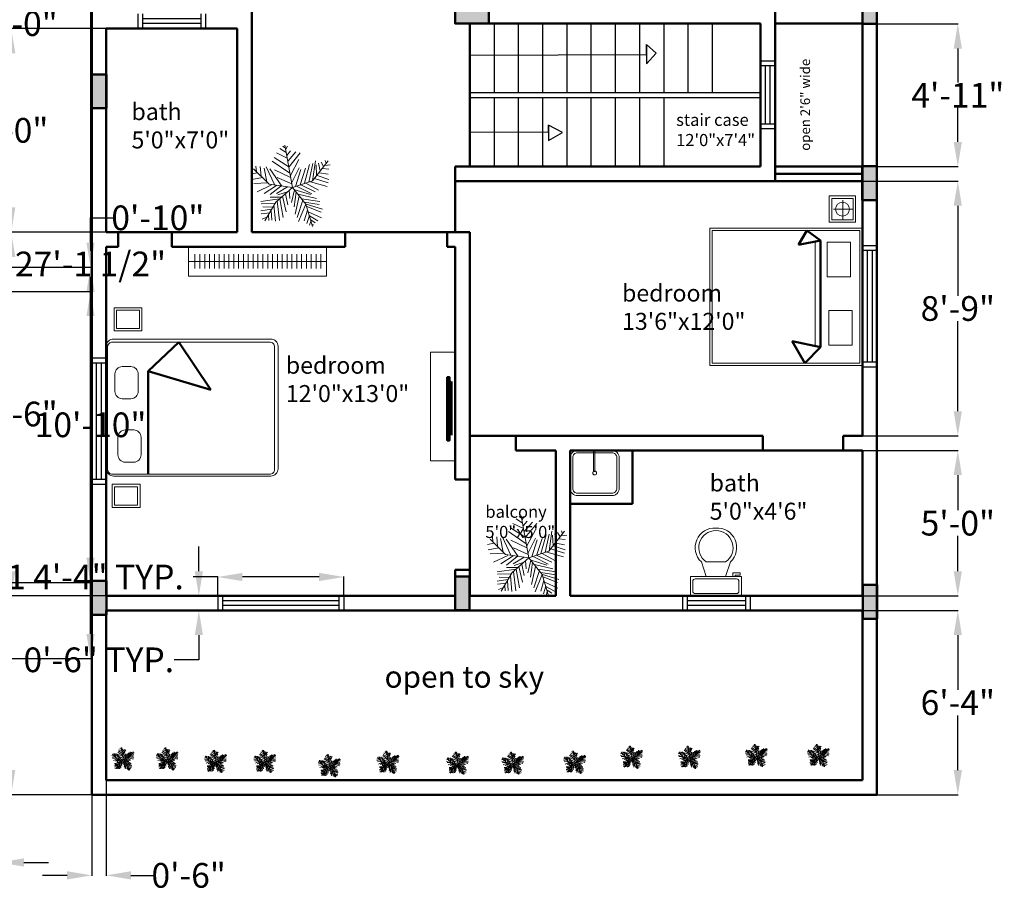
# Model space of a CAD drawing. Units: inches. Extents: x 41 to 5965, y 7 to 3328.
# Tile 2 of 6: x 5442 to 5848, y 1735 to 2098. Entities that reach past the tile are written whole.
import ezdxf

# ---------------------------------------------------------------- set-up
doc = ezdxf.new("R2010")
doc.units = ezdxf.units.IN
doc.header["$MEASUREMENT"] = 0
for name, color, linetype, lineweight in [('A-ANNO-DIMS', 2, 'Continuous', 18), ('A-AREA-IDEN', 3, 'Continuous', 18), ('A-FLOR-FIXT', 9, 'Continuous', 18), ('A-FLOR-STRS', 3, 'Continuous', 25), ('A-FURN', 8, 'Continuous', 18), ('A-GLAZ', 4, 'Continuous', 25), ('A-WALL', 7, 'Continuous', 50), ('A-WALL-PATT', 8, 'Continuous', 13), ('L-PLNT', 82, 'Continuous', 13)]:
    doc.layers.add(name, color=color, linetype=linetype, lineweight=lineweight)
doc.styles.get("Standard").update_dxf_attribs({"font": 'arial.ttf'})
doc.dimstyles.get("Standard").update_dxf_attribs({"dimtxt": 10.18, "dimasz": 10.18, "dimexe": 0.18, "dimexo": 0.0625, "dimgap": 0.09, "dimtad": 0, "dimtih": 1, "dimtoh": 1, "dimdec": 0, "dimzin": 0, "dimdsep": 46, "dimlunit": 3, "dimtxsty": 'Standard', "dimcen": 0.09, "dimadec": 0, "dimazin": 0, "dimtfac": 1, "dimtdec": 0, "dimtofl": 0, "dimtmove": 0, "dimatfit": 3, "dimfxl": 1, "dimtolj": 1, "dimtzin": 0, "dimarcsym": 0})

# ---------------------------------------------------------------- blocks, each defined once
blk = doc.blocks.new('*U6')
for p, q in [((9.5, -6), (9.5, -2)), ((-8, -8.5), (-8, -8)), ((-7, -8), (-7, -9.5)), ((-4, -8), (-6, -14)), ((4, -8), (6, -14)), ((-10, -8.5), (-8, -8.5)), ((-10, -9.5), (-10, -8.5)), ((-7, -9.5), (-10, -9.5)), ((4, -14), (-4, -14))]:
    blk.add_line(p, q)
blk.add_lwpolyline([(10.5, -8), (10.5, 0), (-10.5, 0), (-10.5, -8)], close=True)
for points in [[(-9.5, -2), (-9.5, -6)], [(8.5, -1), (-8.5, -1)], [(-8.5, -7), (8.5, -7)]]:
    blk.add_lwpolyline(points)
for centre, radius, start, end in [((-8.625, -1.875), 0.8839, 81.8699, 188.1301), ((8.625, -1.875), 0.8839, 351.8699, 98.1301), ((-8.625, -6.125), 0.8839, 171.869898, 278.1301), ((8.625, -6.125), 0.8839, 261.8699, 8.1301), ((-0.4772, -19.9188), 8.0953, 133.01722, 273.38), ((0.0374, -19.8731), 7.127, 124.50543, 269.7), ((-0.0373, -19.8731), 7.127, 270.3, 55.4946), ((0.4773, -19.9188), 8.0953, 266.62, 46.9828)]:
    blk.add_arc(centre, radius, start, end)
blk = doc.blocks.new('*U8')
for p, q in [((-10.186, 53.64), (-13.084, 55.962)), ((0, 0), (-10.5, 57)), ((-9.099, 51.782), (-6.563, 55.962)), ((-5.114, 28.097), (-24.676, 40.636)), ((-7.288, 39.707), (-21.778, 46.673)), ((-8.737, 47.138), (-17.069, 52.711)), ((-7.65, 43.423), (-2.578, 49.46)), ((-5.839, 35.992), (4.667, 48.067)), ((-5.114, 27.632), (10.463, 46.673)), ((-48.585, 21.131), (-49.309, 29.026)), ((-43.513, 28.561), (-42.427, 15.558)), ((-35.544, 28.097), (-24.314, 3.947)), ((-3.665, 19.273), (-27.574, 35.527)), ((-2.941, 16.486), (8.652, 37.85)), ((-1.129, 6.734), (9.014, 26.704)), ((16.259, 5.805), (23.142, 31.348)), ((22.055, 7.198), (27.489, 32.277)), ((27, 9), (48, 36)), ((27.127, 9.056), (31.112, 35.992)), ((31.836, 30.883), (32.561, 16.486)), ((35.096, 32.741), (37.27, 22.524)), ((38.719, 34.134), (41.979, 28.561)), ((43.791, 29.954), (51.036, 30.883)), ((44.153, 36.456), (45.239, 32.741)), ((-47.498, 19.737), (-55.83, 18.344)), ((-40.615, 13.7), (-55.105, 10.913)), ((-31.5, 4.5), (-52.5, 25.5)), ((-38.442, 26.239), (-34.819, 7.663)), ((-14.533, 2.09), (-30.834, 25.31)), ((-24.314, 23.917), (-2.941, 13.7)), ((-20.691, 13.7), (-1.129, 4.876)), ((3.942, 1.625), (11.187, 24.381)), ((10.101, 3.483), (17.708, 26.239)), ((33.285, 16.486), (48.862, 10.913)), ((36.183, 19.737), (48.137, 17.88)), ((40.53, 25.775), (48.862, 24.846)), ((-33.37, 6.269), (-52.207, 5.34)), ((-28.299, 3.483), (-47.86, -5.805)), ((-21.416, 3.018), (-38.079, -8.128)), ((0, 0), (-31.5, 4.5)), ((-15.982, 2.09), (-30.11, -9.521)), ((0, 0), (-22.5, -19.5)), ((-6.563, 1.161), (-21.416, -8.128)), ((0, 0), (27, 9)), ((0, 0), (18, -22.5)), ((6.478, 1.625), (26.04, -8.592)), ((11.187, 3.483), (30.749, -5.805)), ((18.07, 5.805), (35.096, -3.483)), ((24.229, 7.663), (46.688, 1.625)), ((29.662, 12.307), (48.137, 6.269)), ((-15.257, -12.772), (-30.11, -12.772)), ((-6.563, -5.805), (-19.967, -9.985)), ((-13.446, -11.378), (-8.737, -32.741)), ((-9.461, -8.592), (-6.201, -23.453)), ((-4.752, -3.483), (-3.665, -14.629)), ((2.493, -3.019), (-1.491, -20.202)), ((1.769, -2.555), (24.229, -9.521)), ((5.029, -6.27), (2.131, -25.775)), ((9.014, -11.378), (3.58, -35.992)), ((7.565, -9.056), (32.198, -14.629)), ((-17.431, -15.094), (-42.789, -18.809)), ((-24.314, -21.596), (-42.427, -22.06)), ((-26.849, -26.24), (-40.253, -25.775)), ((-22.5, -19.5), (-37.5, -45)), ((-25.038, -23.918), (-22.865, -45.281)), ((-20.691, -18.345), (-17.793, -44.352)), ((-17.069, -15.094), (-12.721, -40.172)), ((14.085, -16.951), (6.478, -40.172)), ((18.07, -22.524), (8.289, -45.745)), ((12.274, -15.094), (36.907, -18.809)), ((16.259, -19.738), (36.183, -22.989)), ((18, -22.5), (27, -52.5)), ((18.433, -22.524), (40.53, -29.026)), ((19.157, -25.311), (38.719, -33.206)), ((-28.299, -29.026), (-42.789, -31.348)), ((-30.834, -34.135), (-42.427, -35.528)), ((-34.457, -39.708), (-40.978, -42.494)), ((-32.646, -36.921), (-31.921, -44.352)), ((-29.023, -30.884), (-27.936, -43.887)), ((20.244, -30.419), (15.897, -44.816)), ((22.78, -37.85), (19.519, -48.532)), ((21.331, -32.741), (39.081, -40.636)), ((22.78, -38.314), (34.372, -44.816)), ((24.591, -45.745), (23.142, -50.854)), ((24.591, -43.423), (30.749, -47.603)), ((26.764, -49.925), (28.213, -50.854))]:
    blk.add_line(p, q)
blk = doc.blocks.new('WIN-1200')
for p, q in [((0, 0), (0, 6)), ((2, 0), (2, 6)), ((50, 0), (50, 6)), ((52, 0), (52, 6)), ((2, 4), (50, 4)), ((2, 2), (50, 2))]:
    blk.add_line(p, q)
blk = doc.blocks.new('WIN-600')
for p, q in [((0, 0), (0, 6)), ((2, 0), (2, 6)), ((26, 0), (26, 6)), ((28, 0), (28, 6)), ((2, 4), (26, 4)), ((2, 2), (26, 2))]:
    blk.add_line(p, q)
blk = doc.blocks.new('*D20')
at = {"layer": 'A-ANNO-DIMS', "color": 0, "lineweight": -2, "transparency": 16777216}
for p, q in [((5523.49, 1868.32), (5513.31, 1868.32)), ((5523.49, 1860.58), (5523.49, 1868.5)), ((5565.31, 1868.32), (5533.67, 1868.32)), ((5575.49, 1860.58), (5575.49, 1868.5))]:
    blk.add_line(p, q, dxfattribs=at)
at = {"layer": 'A-ANNO-DIMS', "color": 0, "transparency": 16777216}
for points in [[(5533.67, 1870.02), (5533.67, 1866.62), (5523.49, 1868.32)], [(5565.31, 1870.02), (5565.31, 1866.62), (5575.49, 1868.32)]]:
    blk.add_solid(points, dxfattribs=at)
at = {"layer": 'Defpoints', "color": 0, "transparency": 16777216}
for p in [(5523.49, 1868.32), (5523.49, 1860.52), (5575.49, 1860.52)]:
    blk.add_point(p, dxfattribs=at)
at = {"layer": 'A-ANNO-DIMS', "color": 0, "transparency": 16777216, "insert": (5436.17, 1868.32), "char_height": 10.18, "attachment_point": 5}
blk.add_mtext('\\A1;WINDOW W1 4\'-4" TYP.', dxfattribs=at)
blk = doc.blocks.new('*D21')
at = {"layer": 'A-ANNO-DIMS', "color": 0, "lineweight": -2, "transparency": 16777216}
for p, q in [((5515.69, 1870.7), (5515.69, 1880.88)), ((5523.43, 1860.52), (5515.51, 1860.52)), ((5523.43, 1854.52), (5515.51, 1854.52)), ((5515.69, 1844.34), (5515.69, 1834.16)), ((5515.69, 1834.16), (5505.51, 1834.16))]:
    blk.add_line(p, q, dxfattribs=at)
at = {"layer": 'A-ANNO-DIMS', "color": 0, "transparency": 16777216}
for points in [[(5514, 1870.7), (5517.39, 1870.7), (5515.69, 1860.52)], [(5514, 1844.34), (5517.39, 1844.34), (5515.69, 1854.52)]]:
    blk.add_solid(points, dxfattribs=at)
at = {"layer": 'Defpoints', "color": 0, "transparency": 16777216}
for p in [(5523.49, 1860.52), (5515.69, 1854.52), (5523.49, 1854.52)]:
    blk.add_point(p, dxfattribs=at)
at = {"layer": 'A-ANNO-DIMS', "color": 0, "transparency": 16777216, "insert": (5474.4, 1834.16), "char_height": 10.18, "attachment_point": 5}
blk.add_mtext('\\A1;0\'-6" TYP.', dxfattribs=at)
blk = doc.blocks.new('*D41')
at = {"layer": 'A-ANNO-DIMS', "color": 0, "lineweight": -2, "transparency": 16777216}
for p, q in [((5433.48, 2160.2), (5471.17, 2160.2)), ((5470.99, 2150.02), (5470.99, 2002.77)), ((5470.99, 1844.82), (5470.99, 1992.07)), ((5433.55, 1834.64), (5471.17, 1834.64))]:
    blk.add_line(p, q, dxfattribs=at)
at = {"layer": 'A-ANNO-DIMS', "color": 0, "transparency": 16777216}
for points in [[(5469.29, 2150.02), (5472.69, 2150.02), (5470.99, 2160.2)], [(5469.29, 1844.82), (5472.69, 1844.82), (5470.99, 1834.64)]]:
    blk.add_solid(points, dxfattribs=at)
at = {"layer": 'Defpoints', "color": 0, "transparency": 16777216}
for p in [(5433.42, 2160.2), (5470.99, 2160.2), (5433.49, 1834.64)]:
    blk.add_point(p, dxfattribs=at)
at = {"layer": 'A-ANNO-DIMS', "color": 0, "transparency": 16777216, "insert": (5470.99, 1997.42), "char_height": 10.18, "attachment_point": 5}
blk.add_mtext('\\A1;27\'-1 1/2"', dxfattribs=at)
blk = doc.blocks.new('*D43')
at = {"layer": 'A-ANNO-DIMS', "color": 0, "lineweight": -2, "transparency": 16777216}
for p, q in [((5365.62, 1866.02), (5365.62, 1750.4)), ((5433.3, 1866.02), (5433.3, 1750.4)), ((5355.44, 1750.58), (5345.26, 1750.58)), ((5443.48, 1750.58), (5453.66, 1750.58))]:
    blk.add_line(p, q, dxfattribs=at)
at = {"layer": 'A-ANNO-DIMS', "color": 0, "transparency": 16777216}
for points in [[(5355.44, 1752.28), (5355.44, 1748.89), (5365.62, 1750.58)], [(5443.48, 1752.28), (5443.48, 1748.89), (5433.3, 1750.58)]]:
    blk.add_solid(points, dxfattribs=at)
at = {"layer": 'Defpoints', "color": 0, "transparency": 16777216}
for p in [(5365.62, 1866.08), (5433.3, 1866.08), (5433.3, 1750.58)]:
    blk.add_point(p, dxfattribs=at)
at = {"layer": 'A-ANNO-DIMS', "color": 0, "transparency": 16777216, "insert": (5399.46, 1750.58), "char_height": 10.18, "attachment_point": 5}
blk.add_mtext('\\A1;5\'-7 1/2"', dxfattribs=at)
blk = doc.blocks.new('*D44')
at = {"layer": 'A-ANNO-DIMS', "color": 0, "lineweight": -2, "transparency": 16777216}
for p, q in [((5470.99, 2006.26), (5470.99, 2016.44)), ((5470.99, 2016.44), (5481.17, 2016.44)), ((5433.36, 1996.08), (5471.17, 1996.08)), ((5433.36, 1986.08), (5471.17, 1986.08)), ((5470.99, 1975.9), (5470.99, 1965.72))]:
    blk.add_line(p, q, dxfattribs=at)
at = {"layer": 'A-ANNO-DIMS', "color": 0, "transparency": 16777216}
for points in [[(5469.29, 2006.26), (5472.69, 2006.26), (5470.99, 1996.08)], [(5469.29, 1975.9), (5472.69, 1975.9), (5470.99, 1986.08)]]:
    blk.add_solid(points, dxfattribs=at)
at = {"layer": 'Defpoints', "color": 0, "transparency": 16777216}
for p in [(5433.3, 1996.08), (5470.99, 1996.08), (5433.3, 1986.08)]:
    blk.add_point(p, dxfattribs=at)
at = {"layer": 'A-ANNO-DIMS', "color": 0, "transparency": 16777216, "insert": (5498.75, 2016.44), "char_height": 10.18, "attachment_point": 5}
blk.add_mtext('\\A1;0\'-10"', dxfattribs=at)
blk = doc.blocks.new('*D45')
at = {"layer": 'A-ANNO-DIMS', "color": 0, "lineweight": -2, "transparency": 16777216}
for p, q in [((5365.69, 1996.08), (5471.17, 1996.08)), ((5470.99, 1985.9), (5470.99, 1936.37)), ((5470.99, 1876.26), (5470.99, 1925.79)), ((5365.69, 1866.08), (5471.17, 1866.08))]:
    blk.add_line(p, q, dxfattribs=at)
at = {"layer": 'A-ANNO-DIMS', "color": 0, "transparency": 16777216}
for points in [[(5469.29, 1985.9), (5472.69, 1985.9), (5470.99, 1996.08)], [(5469.29, 1876.26), (5472.69, 1876.26), (5470.99, 1866.08)]]:
    blk.add_solid(points, dxfattribs=at)
at = {"layer": 'Defpoints', "color": 0, "transparency": 16777216}
for p in [(5365.62, 1996.08), (5470.99, 1996.08), (5365.62, 1866.08)]:
    blk.add_point(p, dxfattribs=at)
at = {"layer": 'A-ANNO-DIMS', "color": 0, "transparency": 16777216, "insert": (5470.99, 1931.08), "char_height": 10.18, "attachment_point": 5}
blk.add_mtext('\\A1;10\'-10"', dxfattribs=at)
blk = doc.blocks.new('*D50')
at = {"layer": 'A-ANNO-DIMS', "color": 0, "lineweight": -2, "transparency": 16777216}
for p, q in [((5471.43, 2414.52), (5438.06, 2414.52)), ((5438.24, 2404.34), (5438.24, 2101.81)), ((5438.24, 1788.7), (5438.24, 2091.23)), ((5471.43, 1778.52), (5438.06, 1778.52))]:
    blk.add_line(p, q, dxfattribs=at)
at = {"layer": 'A-ANNO-DIMS', "color": 0, "transparency": 16777216}
for points in [[(5436.55, 2404.34), (5439.94, 2404.34), (5438.24, 2414.52)], [(5436.55, 1788.7), (5439.94, 1788.7), (5438.24, 1778.52)]]:
    blk.add_solid(points, dxfattribs=at)
at = {"layer": 'Defpoints', "color": 0, "transparency": 16777216}
for p in [(5438.24, 2414.52), (5471.49, 2414.52), (5471.49, 1778.52)]:
    blk.add_point(p, dxfattribs=at)
at = {"layer": 'A-ANNO-DIMS', "color": 0, "transparency": 16777216, "insert": (5438.24, 2096.52), "char_height": 10.18, "attachment_point": 5}
blk.add_mtext('\\A1;53\'-0"', dxfattribs=at)
blk = doc.blocks.new('*D51')
at = {"layer": 'A-ANNO-DIMS', "color": 0, "lineweight": -2, "transparency": 16777216}
for p, q in [((5477.49, 1784.46), (5477.49, 1745.09)), ((5471.49, 1778.46), (5471.49, 1745.09)), ((5461.31, 1745.27), (5451.13, 1745.27)), ((5487.67, 1745.27), (5497.85, 1745.27))]:
    blk.add_line(p, q, dxfattribs=at)
at = {"layer": 'A-ANNO-DIMS', "color": 0, "transparency": 16777216}
for points in [[(5461.31, 1746.97), (5461.31, 1743.57), (5471.49, 1745.27)], [(5487.67, 1746.97), (5487.67, 1743.57), (5477.49, 1745.27)]]:
    blk.add_solid(points, dxfattribs=at)
at = {"layer": 'Defpoints', "color": 0, "transparency": 16777216}
for p in [(5477.49, 1784.52), (5471.49, 1778.52), (5477.49, 1745.27)]:
    blk.add_point(p, dxfattribs=at)
at = {"layer": 'A-ANNO-DIMS', "color": 0, "transparency": 16777216, "insert": (5511.47, 1745.27), "char_height": 10.18, "attachment_point": 5}
blk.add_mtext('\\A1;0\'-6"', dxfattribs=at)
blk = doc.blocks.new('*D52')
at = {"layer": 'A-ANNO-DIMS', "color": 0, "lineweight": -2, "transparency": 16777216}
for p, q in [((5789.56, 1854.52), (5829.04, 1854.52)), ((5828.86, 1844.34), (5828.86, 1821.81)), ((5828.86, 1788.7), (5828.86, 1811.23)), ((5795.56, 1778.52), (5829.04, 1778.52))]:
    blk.add_line(p, q, dxfattribs=at)
at = {"layer": 'A-ANNO-DIMS', "color": 0, "transparency": 16777216}
for points in [[(5827.16, 1844.34), (5830.56, 1844.34), (5828.86, 1854.52)], [(5827.16, 1788.7), (5830.56, 1788.7), (5828.86, 1778.52)]]:
    blk.add_solid(points, dxfattribs=at)
at = {"layer": 'Defpoints', "color": 0, "transparency": 16777216}
for p in [(5789.49, 1854.52), (5828.86, 1854.52), (5795.49, 1778.52)]:
    blk.add_point(p, dxfattribs=at)
at = {"layer": 'A-ANNO-DIMS', "color": 0, "transparency": 16777216, "insert": (5828.86, 1816.52), "char_height": 10.18, "attachment_point": 5}
blk.add_mtext('\\A1;6\'-4"', dxfattribs=at)
blk = doc.blocks.new('*D53')
at = {"layer": 'A-ANNO-DIMS', "color": 0, "lineweight": -2, "transparency": 16777216}
for p, q in [((5789.56, 1920.52), (5829.04, 1920.52)), ((5828.86, 1910.34), (5828.86, 1895.81)), ((5828.86, 1870.7), (5828.86, 1885.23)), ((5789.56, 1860.52), (5829.04, 1860.52))]:
    blk.add_line(p, q, dxfattribs=at)
at = {"layer": 'A-ANNO-DIMS', "color": 0, "transparency": 16777216}
for points in [[(5827.16, 1910.34), (5830.56, 1910.34), (5828.86, 1920.52)], [(5827.16, 1870.7), (5830.56, 1870.7), (5828.86, 1860.52)]]:
    blk.add_solid(points, dxfattribs=at)
at = {"layer": 'Defpoints', "color": 0, "transparency": 16777216}
for p in [(5789.49, 1920.52), (5828.86, 1920.52), (5789.49, 1860.52)]:
    blk.add_point(p, dxfattribs=at)
at = {"layer": 'A-ANNO-DIMS', "color": 0, "transparency": 16777216, "insert": (5828.86, 1890.52), "char_height": 10.18, "attachment_point": 5}
blk.add_mtext('\\A1;5\'-0"', dxfattribs=at)
blk = doc.blocks.new('*D54')
at = {"layer": 'A-ANNO-DIMS', "color": 0, "lineweight": -2, "transparency": 16777216}
for p, q in [((5789.56, 2031.57), (5829.04, 2031.57)), ((5828.86, 2021.39), (5828.86, 1984.33)), ((5828.86, 1936.7), (5828.86, 1973.76)), ((5789.56, 1926.52), (5829.04, 1926.52))]:
    blk.add_line(p, q, dxfattribs=at)
at = {"layer": 'A-ANNO-DIMS', "color": 0, "transparency": 16777216}
for points in [[(5827.16, 2021.39), (5830.56, 2021.39), (5828.86, 2031.57)], [(5827.16, 1936.7), (5830.56, 1936.7), (5828.86, 1926.52)]]:
    blk.add_solid(points, dxfattribs=at)
at = {"layer": 'Defpoints', "color": 0, "transparency": 16777216}
for p in [(5789.49, 2031.57), (5828.86, 2031.57), (5789.49, 1926.52)]:
    blk.add_point(p, dxfattribs=at)
at = {"layer": 'A-ANNO-DIMS', "color": 0, "transparency": 16777216, "insert": (5828.86, 1979.04), "char_height": 10.18, "attachment_point": 5}
blk.add_mtext('\\A1;8\'-9"', dxfattribs=at)
blk = doc.blocks.new('*D55')
at = {"layer": 'A-ANNO-DIMS', "color": 0, "lineweight": -2, "transparency": 16777216}
for p, q in [((5789.55, 2096.43), (5829.04, 2096.43)), ((5828.86, 2086.25), (5828.86, 2072.2)), ((5828.86, 2047.75), (5828.86, 2061.8)), ((5789.56, 2037.57), (5829.04, 2037.57))]:
    blk.add_line(p, q, dxfattribs=at)
at = {"layer": 'A-ANNO-DIMS', "color": 0, "transparency": 16777216}
for points in [[(5827.16, 2086.25), (5830.56, 2086.25), (5828.86, 2096.43)], [(5827.16, 2047.75), (5830.56, 2047.75), (5828.86, 2037.57)]]:
    blk.add_solid(points, dxfattribs=at)
at = {"layer": 'Defpoints', "color": 0, "transparency": 16777216}
for p in [(5789.48, 2096.43), (5828.86, 2096.43), (5789.49, 2037.57)]:
    blk.add_point(p, dxfattribs=at)
at = {"layer": 'A-ANNO-DIMS', "color": 0, "transparency": 16777216, "insert": (5828.86, 2067), "char_height": 10.18, "attachment_point": 5}
blk.add_mtext('\\A1;4\'-11"', dxfattribs=at)
blk = doc.blocks.new('*D59')
at = {"layer": 'A-ANNO-DIMS', "color": 0, "lineweight": -2, "transparency": 16777216}
for p, q in [((5477.43, 2010.52), (5438.06, 2010.52)), ((5438.24, 2000.34), (5438.24, 1940.81)), ((5438.24, 1870.7), (5438.24, 1930.23)), ((5477.43, 1860.52), (5438.06, 1860.52))]:
    blk.add_line(p, q, dxfattribs=at)
at = {"layer": 'A-ANNO-DIMS', "color": 0, "transparency": 16777216}
for points in [[(5436.55, 2000.34), (5439.94, 2000.34), (5438.24, 2010.52)], [(5436.55, 1870.7), (5439.94, 1870.7), (5438.24, 1860.52)]]:
    blk.add_solid(points, dxfattribs=at)
at = {"layer": 'Defpoints', "color": 0, "transparency": 16777216}
for p in [(5438.24, 2010.52), (5477.49, 2010.52), (5477.49, 1860.52)]:
    blk.add_point(p, dxfattribs=at)
at = {"layer": 'A-ANNO-DIMS', "color": 0, "transparency": 16777216, "insert": (5438.24, 1935.52), "char_height": 10.18, "attachment_point": 5}
blk.add_mtext('\\A1;12\'-6"', dxfattribs=at)
blk = doc.blocks.new('*D60')
at = {"layer": 'A-ANNO-DIMS', "color": 0, "lineweight": -2, "transparency": 16777216}
for p, q in [((5477.43, 2094.52), (5438.06, 2094.52)), ((5438.24, 2084.34), (5438.24, 2057.81)), ((5438.24, 2020.7), (5438.24, 2047.23)), ((5477.43, 2010.52), (5438.06, 2010.52))]:
    blk.add_line(p, q, dxfattribs=at)
at = {"layer": 'A-ANNO-DIMS', "color": 0, "transparency": 16777216}
for points in [[(5436.55, 2084.34), (5439.94, 2084.34), (5438.24, 2094.52)], [(5436.55, 2020.7), (5439.94, 2020.7), (5438.24, 2010.52)]]:
    blk.add_solid(points, dxfattribs=at)
at = {"layer": 'Defpoints', "color": 0, "transparency": 16777216}
for p in [(5438.24, 2094.52), (5477.49, 2094.52), (5477.49, 2010.52)]:
    blk.add_point(p, dxfattribs=at)
at = {"layer": 'A-ANNO-DIMS', "color": 0, "transparency": 16777216, "insert": (5438.24, 2052.52), "char_height": 10.18, "attachment_point": 5}
blk.add_mtext('\\A1;7\'-0"', dxfattribs=at)

msp = doc.modelspace()

# ---------------------------------------------------------------- hatches: boundary and pattern name
at = {"layer": 'A-WALL-PATT'}
h = msp.add_hatch(color=256, dxfattribs=at)
h.dxf.hatch_style = 1
h.paths.add_polyline_path([(5477.49, 2378.52), (5471.49, 2378.52), (5471.49, 2364.59), (5477.49, 2364.59)])
h.paths.add_polyline_path([(5627.49, 2372.52), (5627.52, 2378.52), (5621.52, 2378.52), (5621.52, 2364.59), (5627.49, 2364.59)])
h.paths.add_polyline_path([(5795.41, 2378.41), (5789.41, 2378.41), (5789.41, 2372.52), (5789.49, 2372.52), (5789.49, 2364.48), (5795.41, 2364.48)])
h.paths.add_polyline_path([(5485.48, 2284.52), (5477.49, 2284.52), (5471.55, 2284.61), (5471.55, 2278.61), (5485.48, 2278.61)])
h.paths.add_polyline_path([(5477.49, 2075.53), (5471.54, 2075.53), (5471.54, 2061.6), (5477.49, 2061.6)])
h.paths.add_polyline_path([(5477.49, 1860.52), (5477.49, 1866.7), (5471.52, 1866.7), (5471.52, 1852.76), (5477.49, 1852.76), (5477.49, 1854.52), (5477.51, 1860.52)])
h.paths.add_polyline_path([(5627.43, 1868.54), (5621.49, 1868.54), (5621.49, 1860.52), (5621.43, 1854.61), (5627.43, 1854.61)])
h.paths.add_polyline_path([(5795.49, 1865.02), (5789.61, 1865.02), (5789.61, 1851.08), (5795.49, 1851.08)])
h.paths.add_polyline_path([(5795.48, 2110.36), (5789.49, 2110.36), (5789.49, 2102.64), (5789.49, 2096.43), (5795.48, 2096.43)])
h.paths.add_polyline_path([(5795.4, 2037.71), (5789.49, 2037.71), (5789.49, 2031.57), (5789.49, 2023.78), (5795.4, 2023.78)])
h.paths.add_polyline_path([(5635.41, 2102.54), (5621.49, 2102.54), (5621.49, 2096.64), (5627.49, 2096.64), (5635.41, 2096.64)])

# ---------------------------------------------------------------- linework, layer by layer
at = {"layer": 'A-FLOR-FIXT'}
for points in [[(5668.95, 1917.52, -0.414214), (5671.95, 1920.52), (5686.14, 1920.52, -0.414214), (5689.14, 1917.52), (5689.14, 1904.86, -0.414214), (5686.14, 1901.86), (5671.95, 1901.86, -0.414214), (5668.95, 1904.86)], [(5669.95, 1917.52, -0.414214), (5671.95, 1919.52), (5686.14, 1919.52, -0.414214), (5688.14, 1917.52), (5688.14, 1904.86, -0.414214), (5686.14, 1902.86), (5671.95, 1902.86, -0.414214), (5669.95, 1904.86)]]:
    msp.add_lwpolyline(points, format="xyb", close=True, dxfattribs=at)
msp.add_lwpolyline([(5679.05, 1920.52), (5679.05, 1920.52), (5678.56, 1920.52), (5678.56, 1920.52), (5678.56, 1911.81), (5678.56, 1911.81), (5679.05, 1911.81), (5679.05, 1911.81)], close=True, dxfattribs=at)
msp.add_circle((5679.05, 1911.19), 0.791, dxfattribs=at)
at = {"layer": 'A-FLOR-STRS'}
for p, q in [((5637.49, 2096.64), (5637.49, 2068.1)), ((5647.49, 2096.64), (5647.49, 2068.1)), ((5657.49, 2096.64), (5657.49, 2068.1)), ((5657.49, 2096.64), (5657.49, 2068.1)), ((5667.49, 2096.64), (5667.49, 2068.1)), ((5677.49, 2096.64), (5677.49, 2068.1)), ((5687.49, 2096.64), (5687.49, 2068.1)), ((5697.49, 2096.64), (5697.49, 2068.1)), ((5707.49, 2096.64), (5707.49, 2068.1)), ((5717.49, 2096.64), (5717.49, 2068.1)), ((5727.49, 2096.64), (5727.49, 2068.1)), ((5700.36, 2083.73), (5700.35, 2087.9)), ((5700.35, 2087.9), (5700.37, 2079.99)), ((5704.45, 2084.33), (5700.35, 2087.9)), ((5700.37, 2079.99), (5704.45, 2084.33)), ((5627.49, 2083.54), (5700.36, 2083.73)), ((5627.49, 2068.1), (5747.49, 2068.1)), ((5627.49, 2066.1), (5747.49, 2066.1)), ((5637.49, 2066.1), (5637.49, 2037.57)), ((5647.49, 2066.1), (5647.49, 2037.57)), ((5657.49, 2066.1), (5657.49, 2037.57)), ((5657.49, 2066.1), (5657.49, 2037.57)), ((5667.49, 2066.1), (5667.49, 2037.57)), ((5677.49, 2066.1), (5677.49, 2037.57)), ((5687.49, 2066.1), (5687.49, 2037.57)), ((5697.49, 2066.1), (5697.49, 2037.57)), ((5707.49, 2066.1), (5707.49, 2037.57)), ((5627.49, 2051.8), (5660.03, 2051.91)), ((5660.03, 2051.91), (5660.03, 2054.68)), ((5660.03, 2054.68), (5660.03, 2048.36)), ((5665.7, 2051.63), (5660.03, 2054.68)), ((5660.03, 2048.36), (5665.7, 2051.63))]:
    msp.add_line(p, q, dxfattribs=at)
at = {"layer": 'A-FURN'}
for p, q in [((5781.48, 2023.67), (5781.48, 2015.6)), ((5777.56, 2020.03), (5785.36, 2019.99)), ((5769.97, 2006.64), (5770.01, 1963.52)), ((5514.09, 2001.39), (5514.09, 1995.54)), ((5516.09, 2001.39), (5516.09, 1995.54)), ((5518.09, 2001.39), (5518.09, 1995.54)), ((5520.09, 2001.39), (5520.09, 1995.54)), ((5522.09, 2001.39), (5522.09, 1995.54)), ((5524.09, 2001.39), (5524.09, 1995.54)), ((5526.09, 2001.39), (5526.09, 1995.54)), ((5528.09, 2001.39), (5528.09, 1995.54)), ((5530.09, 2001.39), (5530.09, 1995.54)), ((5532.09, 2001.39), (5532.09, 1995.54)), ((5534.09, 2001.39), (5534.09, 1995.54)), ((5536.09, 2001.39), (5536.09, 1995.54)), ((5538.09, 2001.39), (5538.09, 1995.54)), ((5540.09, 2001.39), (5540.09, 1995.54)), ((5542.09, 2001.39), (5542.09, 1995.54)), ((5544.09, 2001.39), (5544.09, 1995.54)), ((5546.09, 2001.39), (5546.09, 1995.54)), ((5548.09, 2001.39), (5548.09, 1995.54)), ((5550.09, 2001.39), (5550.09, 1995.54)), ((5552.09, 2001.39), (5552.09, 1995.54)), ((5554.09, 2001.39), (5554.09, 1995.54)), ((5556.09, 2001.39), (5556.09, 1995.54)), ((5558.09, 2001.39), (5558.09, 1995.54)), ((5560.09, 2001.39), (5560.09, 1995.54)), ((5562.09, 2001.39), (5562.09, 1995.54)), ((5564.09, 2001.39), (5564.09, 1995.54)), ((5566.09, 2001.39), (5566.09, 1995.54)), ((5511.37, 1998.46), (5568.37, 1998.46))]:
    msp.add_line(p, q, dxfattribs=at)
for points in [[(5775.82, 2025.47), (5786.71, 2025.47), (5786.71, 2014.6), (5775.82, 2014.6)], [(5776.82, 2024.47), (5785.71, 2024.47), (5785.71, 2015.6), (5776.82, 2015.6)], [(5789.49, 2012.2), (5726.51, 2012.2), (5726.51, 1955.56), (5789.49, 1955.56)], [(5788.49, 2011.2), (5727.51, 2011.2), (5727.51, 1956.56), (5788.49, 1956.56)], [(5511.37, 2004.52), (5511.37, 2004.52), (5568.37, 2004.52), (5568.37, 2004.52), (5568.37, 1992.4), (5568.37, 1992.4), (5511.37, 1992.4), (5511.37, 1992.4)], [(5774.97, 2006.44), (5784.53, 2006.44), (5784.53, 1992.05), (5774.97, 1992.05)], [(5480.7, 1979.36), (5480.7, 1979.36), (5492.22, 1979.36), (5492.22, 1979.36), (5492.22, 1969.77), (5492.22, 1969.77), (5480.7, 1969.77), (5480.7, 1969.77)], [(5481.7, 1978.36), (5491.22, 1978.36), (5491.22, 1970.77), (5481.7, 1970.77)], [(5775.68, 1978.28), (5785.24, 1978.28), (5785.24, 1963.89), (5775.68, 1963.89)], [(5621.49, 1961.01), (5621.49, 1961.01), (5611.31, 1961.01), (5611.31, 1961.01), (5611.31, 1916.22), (5611.31, 1916.22), (5621.49, 1916.22), (5621.49, 1916.22)], [(5479.89, 1906.54), (5479.89, 1906.54), (5491.41, 1906.54), (5491.41, 1906.54), (5491.41, 1896.96), (5491.41, 1896.96), (5479.89, 1896.96), (5479.89, 1896.96)], [(5480.89, 1905.54), (5490.41, 1905.54), (5490.41, 1897.96), (5480.89, 1897.96)]]:
    msp.add_lwpolyline(points, close=True, dxfattribs=at)
for points in [[(5477.49, 1963.44, -0.414214), (5480.49, 1966.44), (5545.35, 1966.44, -0.414214), (5548.35, 1963.44), (5548.35, 1912.92, -0.414214), (5545.35, 1909.92), (5480.49, 1909.92, -0.414214), (5477.49, 1912.92)], [(5478.04, 1963.17, -0.414214), (5480.04, 1965.17), (5544.9, 1965.17, -0.414214), (5546.9, 1963.17), (5546.9, 1912.66, -0.414214), (5544.9, 1910.66), (5480.04, 1910.66, -0.414214), (5478.04, 1912.66)], [(5481.08, 1952.1, -0.414214), (5484.08, 1955.1), (5487.65, 1955.1, -0.414214), (5490.65, 1952.1), (5490.65, 1944.81, -0.414214), (5487.65, 1941.81), (5484.08, 1941.81, -0.414214), (5481.08, 1944.81)], [(5482.28, 1925.97, -0.414214), (5485.28, 1928.97), (5488.85, 1928.97, -0.414214), (5491.85, 1925.97), (5491.85, 1918.68, -0.414214), (5488.85, 1915.68), (5485.28, 1915.68, -0.414214), (5482.28, 1918.68)]]:
    msp.add_lwpolyline(points, format="xyb", close=True, dxfattribs=at)
msp.add_circle((5781.27, 2020.03), 2.88, dxfattribs=at)
at = {"layer": 'A-GLAZ'}
for p, q in [((5789.49, 2005.04), (5795.49, 2005.04)), ((5789.49, 2003.04), (5795.49, 2003.04)), ((5791.49, 2003.04), (5791.49, 1957.04)), ((5793.49, 2003.04), (5793.49, 1957.04)), ((5789.49, 1957.04), (5795.49, 1957.04)), ((5789.49, 1955.04), (5795.49, 1955.04))]:
    msp.add_line(p, q, dxfattribs=at)
at = {"layer": 'A-WALL'}
for p, q in [((5471.49, 1778.52), (5471.49, 2378.52)), ((5795.49, 2378.52), (5795.49, 1778.52)), ((5537.49, 2278.52), (5537.49, 2010.52)), ((5621.49, 2278.52), (5621.49, 2096.64)), ((5753.49, 2096.64), (5753.49, 2102.64)), ((5789.49, 2102.64), (5789.49, 2096.64)), ((5621.49, 2096.64), (5627.49, 2096.64)), ((5627.49, 2096.64), (5747.49, 2096.64)), ((5627.49, 2096.64), (5627.49, 2037.57)), ((5747.49, 2096.64), (5747.49, 2037.57)), ((5753.49, 2096.64), (5753.49, 2037.57)), ((5753.49, 2096.64), (5789.49, 2096.64)), ((5789.49, 2096.64), (5789.49, 2037.57)), ((5477.49, 2094.52), (5531.49, 2094.52)), ((5477.49, 2010.52), (5477.49, 2094.52)), ((5531.49, 2094.52), (5531.49, 2010.52)), ((5621.49, 2037.57), (5747.49, 2037.57)), ((5621.49, 2010.52), (5621.49, 2037.57)), ((5753.49, 2037.57), (5789.49, 2037.57)), ((5753.49, 2037.57), (5753.49, 2031.57)), ((5789.49, 2037.57), (5789.49, 2031.57)), ((5627.49, 2031.57), (5621.49, 2031.57)), ((5627.49, 2031.57), (5789.49, 2031.57)), ((5753.49, 2034.57), (5789.49, 2034.57)), ((5789.49, 2031.57), (5789.49, 1926.52)), ((5766.51, 2011.2), (5763.13, 2005.35)), ((5772.22, 2007.07), (5766.51, 2011.2)), ((5477.49, 2010.52), (5531.49, 2010.52)), ((5482.33, 2010.52), (5482.33, 2004.52)), ((5504.49, 2010.52), (5504.49, 2004.52)), ((5537.49, 2010.52), (5621.49, 2010.52)), ((5576.03, 2010.52), (5576.03, 2004.52)), ((5618.11, 2010.52), (5618.11, 2004.52)), ((5621.49, 2010.52), (5627.49, 2010.52)), ((5627.49, 1926.52), (5627.49, 2010.52)), ((5477.49, 2004.52), (5482.33, 2004.52)), ((5477.49, 1860.52), (5477.49, 2004.52)), ((5504.49, 2004.52), (5576.03, 2004.52)), ((5618.11, 2004.52), (5621.49, 2004.52)), ((5621.49, 1908.5), (5621.49, 2004.52)), ((5763.13, 2005.35), (5772.22, 2007.07)), ((5772.22, 2007.07), (5772.22, 1963.03)), ((5494.84, 1953.16), (5507.44, 1965.17)), ((5507.44, 1965.17), (5520.68, 1945.45)), ((5765.8, 1956.56), (5760.57, 1965.62)), ((5760.57, 1965.62), (5772.22, 1963.03)), ((5772.22, 1963.03), (5765.8, 1956.56)), ((5494.84, 1910.66), (5494.84, 1953.16)), ((5520.68, 1945.45), (5494.84, 1953.16)), ((5619.12, 1947.86), (5619.88, 1948.88)), ((5619.88, 1948.88), (5619.88, 1926.74)), ((5619.88, 1926.74), (5619.12, 1928.65)), ((5627.49, 1926.52), (5748.37, 1926.52)), ((5627.49, 1926.52), (5627.49, 1920.52)), ((5646.44, 1926.52), (5646.44, 1920.52)), ((5748.37, 1926.52), (5748.37, 1920.52)), ((5781.59, 1926.52), (5781.59, 1920.52)), ((5781.59, 1926.52), (5789.49, 1926.52)), ((5627.49, 1860.52), (5627.49, 1920.52)), ((5646.44, 1920.52), (5662.95, 1920.52)), ((5662.95, 1860.52), (5662.95, 1920.52)), ((5668.95, 1860.52), (5668.95, 1920.52)), ((5668.95, 1920.52), (5789.49, 1920.52)), ((5694.59, 1920.52), (5694.59, 1898.48)), ((5789.49, 1920.52), (5789.49, 1860.52)), ((5627.49, 1908.5), (5621.49, 1908.5)), ((5694.59, 1898.48), (5668.95, 1898.48)), ((5621.49, 1860.52), (5621.49, 1871.32)), ((5621.49, 1871.32), (5627.49, 1871.32)), ((5477.49, 1860.52), (5621.49, 1860.52)), ((5627.49, 1860.52), (5662.95, 1860.52)), ((5668.95, 1860.52), (5789.49, 1860.52)), ((5477.49, 1784.52), (5477.49, 1854.52)), ((5477.49, 1854.52), (5621.49, 1854.52)), ((5621.49, 1854.52), (5627.49, 1854.52)), ((5627.49, 1854.52), (5789.49, 1854.52)), ((5789.49, 1854.52), (5789.49, 1784.52)), ((5621.49, 1784.52), (5477.49, 1784.52)), ((5621.49, 1784.52), (5627.49, 1784.52)), ((5789.49, 1784.52), (5627.49, 1784.52)), ((5795.49, 1778.52), (5471.49, 1778.52))]:
    msp.add_line(p, q, dxfattribs=at)
for points in [[(5789.48, 2110.36), (5795.48, 2110.36), (5795.48, 2096.43), (5789.48, 2096.43)], [(5635.41, 2102.54), (5635.41, 2096.54), (5621.48, 2096.54), (5621.48, 2102.54)], [(5471.54, 2075.53), (5477.54, 2075.53), (5477.54, 2061.6), (5471.54, 2061.6)], [(5789.4, 2037.71), (5795.4, 2037.71), (5795.4, 2023.78), (5789.4, 2023.78)], [(5619.12, 1950.72), (5619.12, 1950.72), (5618.22, 1950.72), (5618.22, 1950.72), (5618.22, 1924.63), (5618.22, 1924.63), (5619.12, 1924.63), (5619.12, 1924.63)], [(5471.52, 1866.7), (5477.52, 1866.7), (5477.52, 1852.76), (5471.52, 1852.76)], [(5621.43, 1868.54), (5627.43, 1868.54), (5627.43, 1854.61), (5621.43, 1854.61)], [(5789.61, 1865.02), (5795.61, 1865.02), (5795.61, 1851.08), (5789.61, 1851.08)]]:
    msp.add_lwpolyline(points, close=True, dxfattribs=at)

# ---------------------------------------------------------------- block references
at = {"layer": 'A-FLOR-FIXT', "rotation": 180}
msp.add_blockref('*U6', (5729.05, 1860.52), dxfattribs=at)
at = {"layer": 'A-GLAZ'}
for name, p, rotation in [('WIN-600', (5518.49, 2100.52), 180), ('WIN-600', (5753.49, 2053.1), 89.99999999999937), ('WIN-1200', (5477.49, 1906.52), 89.99999999999797), ('WIN-1200', (5575.49, 1860.52), 180), ('WIN-600', (5743.22, 1860.52), 180)]:
    msp.add_blockref(name, p, dxfattribs=dict(at, rotation=rotation))
at = {"layer": 'L-PLNT'}
for p, xscale, yscale, zscale in [((5554.34, 2028.91), 0.3056693623898039, 0.3056693623898039, 0.3056693623898039), ((5651.89, 1876.17), 0.3056693623898039, 0.3056693623898039, 0.3056693623898039), ((5484.6, 1793.08), 0.0860075486317361, 0.0860075486317361, 0.0860075486317361), ((5502.81, 1793.08), 0.0860075486317361, 0.0860075486317361, 0.0860075486317361), ((5522.79, 1792.03), 0.0860075486317361, 0.0860075486317361, 0.0860075486317361), ((5543.11, 1792.03), 0.0860075486317361, 0.0860075486317361, 0.0860075486317361), ((5593.91, 1791.68), 0.0860075486317361, 0.0860075486317361, 0.0860075486317361), ((5622.64, 1791.33), 0.0860075486317361, 0.0860075486317361, 0.0860075486317361), ((5645.42, 1791.33), 0.0860075486317361, 0.0860075486317361, 0.0860075486317361), ((5670.99, 1791.68), 0.0860075486317361, 0.0860075486317361, 0.0860075486317361), ((5694.47, 1793.78), 0.0860075486317361, 0.0860075486317361, 0.0860075486317361), ((5718.29, 1793.78), 0.0860075486317361, 0.0860075486317361, 0.0860075486317361), ((5745.97, 1794.48), 0.0860075486317361, 0.0860075486317361, 0.0860075486317361), ((5771.55, 1794.48), 0.0860075486317361, 0.0860075486317361, 0.0860075486317361), ((5569.74, 1790.28), 0.0860075486317361, 0.0860075486317361, 0.0860075486317361)]:
    msp.add_blockref('*U8', p, dxfattribs=dict(at, xscale=xscale, yscale=yscale, zscale=zscale))

# ---------------------------------------------------------------- texts
at = {"layer": 'A-AREA-IDEN', "insert": (5763.89, 2044.08), "char_height": 4, "attachment_point": 1, "rotation": 90}
msp.add_mtext_dynamic_manual_height_columns('open 2\'6" wide', width=81.0237, gutter_width=1, heights=[0], dxfattribs=at)
at = {"layer": 'A-AREA-IDEN', "attachment_point": 1}
for s, width, insert, char_height in [('bath\\P5\'0"x7\'0"', 52.5564, (5487.89, 2063.73), 7), ('stair case\\P12\'0"x7\'4"', 52.5564, (5712.63, 2059.35), 5), ('bedroom\\P13\'6"x12\'0"', 52.5564, (5690.32, 1988.91), 7), ('bedroom\\P12\'0"x13\'0"', 52.5564, (5551.59, 1959.14), 7), ('bath\\P5\'0"x4\'6"', 52.5564, (5726.48, 1910.61), 7), ('balcony\\P5\'0"x5\'0"', 52.5564, (5633.91, 1897.73), 5), ('open to sky', 81.7364, (5592.32, 1831.66), 9)]:
    msp.add_mtext_dynamic_manual_height_columns(s, width=width, gutter_width=1, heights=[0], dxfattribs=dict(at, insert=insert, char_height=char_height))

# ---------------------------------------------------------------- dimensions: what is measured, and where the dimension line sits
at = {"layer": 'A-ANNO-DIMS'}
for base, p1, p2, picture, middle in [((5438.24, 2414.52), (5471.49, 1778.52), (5471.49, 2414.52), '*D50', (5438.24, 2096.52)), ((5470.99, 2160.2), (5433.49, 1834.64), (5433.42, 2160.2), '*D41', (5470.99, 1997.42)), ((5438.24, 2094.52), (5477.49, 2010.52), (5477.49, 2094.52), '*D60', (5438.24, 2052.52)), ((5828.86, 2096.43), (5789.49, 2037.57), (5789.48, 2096.43), '*D55', (5828.86, 2067)), ((5828.8596, 2031.5679), (5789.4943, 1926.5193), (5789.4943, 2031.5679), '*D54', (5828.8596, 1979.0436)), ((5470.99, 1996.08), (5433.3, 1986.08), (5433.3, 1996.08), '*D44', (5498.75, 2016.44)), ((5438.24, 2010.52), (5477.49, 1860.52), (5477.49, 2010.52), '*D59', (5438.24, 1935.52)), ((5470.99, 1996.08), (5365.62, 1866.08), (5365.62, 1996.08), '*D45', (5470.99, 1931.08)), ((5828.86, 1920.52), (5789.49, 1860.52), (5789.49, 1920.52), '*D53', (5828.86, 1890.52)), ((5828.86, 1854.52), (5795.49, 1778.52), (5789.49, 1854.52), '*D52', (5828.86, 1816.52))]:
    dim = msp.add_linear_dim(base=base, p1=p1, p2=p2, angle=90, dimstyle='Standard', override={"dimdec": 1, "dimlfac": 1, "dimrnd": 0, "dimzin": 1, "dimdsep": 46, "dimlunit": 4, "dimfrac": 2}, dxfattribs=at)
    dim.commit()
    dim.dimension.update_dxf_attribs({"geometry": picture, "text_midpoint": middle})
for base, p1, p2, angle, text, picture, middle in [((5523.49, 1868.32), (5575.49, 1860.52), (5523.49, 1860.52), 180, 'WINDOW W1 <> TYP.', '*D20', (5436.17, 1868.32)), ((5515.69, 1854.52), (5523.49, 1860.52), (5523.49, 1854.52), 270, '<> TYP.', '*D21', (5474.4, 1834.16))]:
    dim = msp.add_linear_dim(base=base, p1=p1, p2=p2, angle=angle, text=text, dimstyle='Standard', override={"dimdec": 1, "dimrnd": 0, "dimzin": 1, "dimlunit": 4, "dimfrac": 2}, dxfattribs=at)
    dim.commit()
    dim.dimension.update_dxf_attribs({"geometry": picture, "text_midpoint": middle})
for base, p1, p2, picture, middle in [((5433.3, 1750.58), (5365.62, 1866.08), (5433.3, 1866.08), '*D43', (5399.46, 1750.58)), ((5477.49, 1745.27), (5471.49, 1778.52), (5477.49, 1784.52), '*D51', (5511.47, 1745.27))]:
    dim = msp.add_linear_dim(base=base, p1=p1, p2=p2, dimstyle='Standard', override={"dimdec": 1, "dimlfac": 1, "dimrnd": 0, "dimzin": 1, "dimdsep": 46, "dimlunit": 4, "dimfrac": 2}, dxfattribs=at)
    dim.commit()
    dim.dimension.update_dxf_attribs({"geometry": picture, "text_midpoint": middle})

doc.saveas('drawing.dxf')
